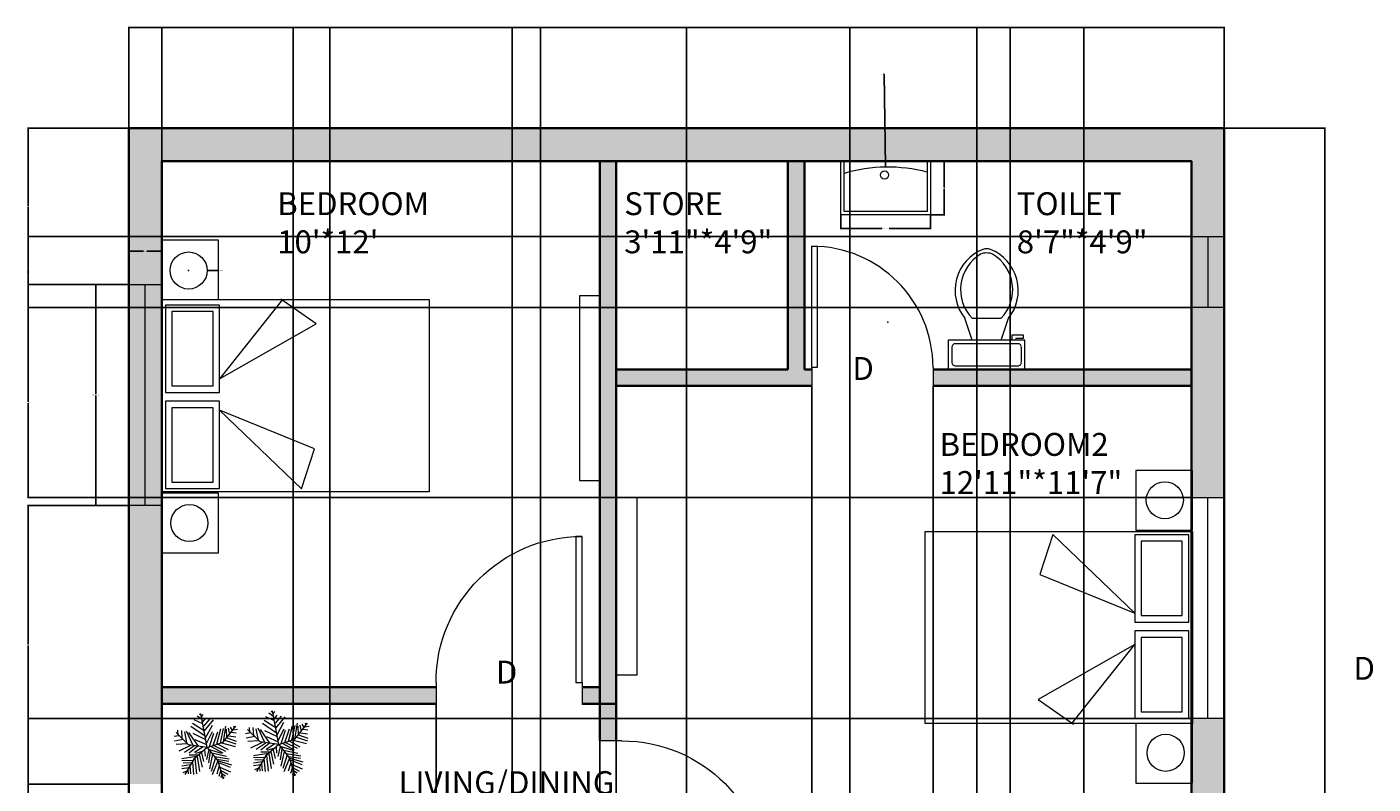
# Model space of a CAD drawing. Units: inches. Extents: x 1841 to 2210, y 2173 to 2736.
# Tile 4 of 4: x 1841 to 2210, y 2529 to 2736. Entities that reach past the tile are written whole.
import ezdxf

# ---------------------------------------------------------------- set-up
doc = ezdxf.new("R2010")
doc.units = ezdxf.units.IN
for name, color, linetype, lineweight in [('A-ANNO-DIMS', 2, 'Continuous', 18), ('A-AREA-IDEN', 10, 'Continuous', 18), ('A-FLOR-FIXT', 9, 'Continuous', 18), ('A-FURN', 8, 'Continuous', 18), ('A-WALL', 7, 'Continuous', 35), ('A-WALL-PATT', 252, 'Continuous', 13), ('BED', 120, 'Continuous', 18), ('DOOR', 50, 'Continuous', 18), ('TEXT', 10, 'Continuous', 18), ('TREE', 70, 'Continuous', 13), ('WIN', 193, 'Continuous', 18)]:
    doc.layers.add(name, color=color, linetype=linetype, lineweight=lineweight)
doc.styles.get("Standard").update_dxf_attribs({"font": 'arial.ttf'})
doc.dimstyles.get("Standard").update_dxf_attribs({"dimtxt": 0.18, "dimasz": 0.18, "dimexe": 0.18, "dimexo": 0.0625, "dimgap": 0.09, "dimtad": 0, "dimtih": 1, "dimtoh": 1, "dimdec": 4, "dimzin": 0, "dimdsep": 46, "dimtxsty": 'Standard', "dimcen": 0.09, "dimadec": 0, "dimazin": 0, "dimtfac": 1, "dimtdec": 4, "dimtofl": 0, "dimtmove": 0, "dimatfit": 3, "dimfxl": 1, "dimtolj": 1, "dimtzin": 0, "dimarcsym": 0})

# ---------------------------------------------------------------- blocks, each defined once
blk = doc.blocks.new('*U2')
for p, q in [((0, 0), (0, -6)), ((40, 0), (40, -6))]:
    blk.add_line(p, q)
blk.add_lwpolyline([(0, 0), (0, 40), (1.75, 40), (1.75, 0)], close=True)
blk.add_arc((0, 0), 40, 0, 90)
blk = doc.blocks.new('*U4')
for p, q in [((9.5, -6), (9.5, -2)), ((-10, -8.5), (-8, -8.5)), ((-10, -9.5), (-10, -8.5)), ((-7, -9.5), (-10, -9.5)), ((-8, -8.5), (-8, -8)), ((-7, -8), (-7, -9.5)), ((-4, -8), (-6, -14)), ((4, -8), (6, -14)), ((4, -14), (-4, -14))]:
    blk.add_line(p, q)
blk.add_lwpolyline([(10.5, -8), (10.5, 0), (-10.5, 0), (-10.5, -8)], close=True)
for points in [[(-9.5, -2), (-9.5, -6)], [(8.5, -1), (-8.5, -1)], [(-8.5, -7), (8.5, -7)]]:
    blk.add_lwpolyline(points)
for centre, radius, start, end in [((-8.62, -1.88), 0.884, 81.8699, 188.1301), ((8.62, -1.88), 0.884, 351.8699, 98.1301), ((-8.62, -6.12), 0.884, 171.8699, 278.1301), ((8.62, -6.12), 0.884, 261.8699, 8.1301), ((3.52, -21.58), 12.17, 141.4691, 247.9714), ((4.2, -21.82), 11.33, 136.3677, 238.9468), ((-3.52, -21.58), 12.17, 292.0284, 38.5307), ((-4.2, -21.82), 11.33, 301.053, 43.6321), ((0, -27.88), 4, 245.7318, 294.2682), ((0, -29), 4, 254.8605, 285.1395)]:
    blk.add_arc(centre, radius, start, end)
blk = doc.blocks.new('*U6')
for p, q in [((-7.288, 39.707), (-21.778, 46.673)), ((-8.737, 47.138), (-17.069, 52.711)), ((-10.186, 53.64), (-13.084, 55.962)), ((0, 0), (-10.5, 57)), ((-9.099, 51.782), (-6.563, 55.962)), ((-7.65, 43.423), (-2.578, 49.46)), ((-5.839, 35.992), (4.667, 48.067)), ((-5.114, 27.632), (10.463, 46.673)), ((-31.5, 4.5), (-52.5, 25.5)), ((-48.585, 21.131), (-49.309, 29.026)), ((-43.513, 28.561), (-42.427, 15.558)), ((-38.442, 26.239), (-34.819, 7.663)), ((-35.544, 28.097), (-24.314, 3.947)), ((-14.533, 2.09), (-30.834, 25.31)), ((-3.665, 19.273), (-27.574, 35.527)), ((-5.114, 28.097), (-24.676, 40.636)), ((-24.314, 23.917), (-2.941, 13.7)), ((-2.941, 16.486), (8.652, 37.85)), ((-1.129, 6.734), (9.014, 26.704)), ((3.942, 1.625), (11.187, 24.381)), ((10.101, 3.483), (17.708, 26.239)), ((16.259, 5.805), (23.142, 31.348)), ((22.055, 7.198), (27.489, 32.277)), ((27, 9), (48, 36)), ((27.127, 9.056), (31.112, 35.992)), ((31.836, 30.883), (32.561, 16.486)), ((35.096, 32.741), (37.27, 22.524)), ((38.719, 34.134), (41.979, 28.561)), ((40.53, 25.775), (48.862, 24.846)), ((43.791, 29.954), (51.036, 30.883)), ((44.153, 36.456), (45.239, 32.741)), ((-47.498, 19.737), (-55.83, 18.344)), ((-40.615, 13.7), (-55.105, 10.913)), ((-33.37, 6.269), (-52.207, 5.34)), ((-28.299, 3.483), (-47.86, -5.805)), ((-21.416, 3.018), (-38.079, -8.128)), ((0, 0), (-31.5, 4.5)), ((-15.982, 2.09), (-30.11, -9.521)), ((0, 0), (-22.5, -19.5)), ((-6.563, 1.161), (-21.416, -8.128)), ((-20.691, 13.7), (-1.129, 4.876)), ((0, 0), (27, 9)), ((0, 0), (18, -22.5)), ((6.478, 1.625), (26.04, -8.592)), ((11.187, 3.483), (30.749, -5.805)), ((18.07, 5.805), (35.096, -3.483)), ((24.229, 7.663), (46.688, 1.625)), ((29.662, 12.307), (48.137, 6.269)), ((33.285, 16.486), (48.862, 10.913)), ((36.183, 19.737), (48.137, 17.88)), ((-17.431, -15.094), (-42.789, -18.809)), ((-24.314, -21.596), (-42.427, -22.06)), ((-22.5, -19.5), (-37.5, -45)), ((-15.257, -12.772), (-30.11, -12.772)), ((-20.691, -18.345), (-17.793, -44.352)), ((-6.563, -5.805), (-19.967, -9.985)), ((-17.069, -15.094), (-12.721, -40.172)), ((-13.446, -11.378), (-8.737, -32.741)), ((-9.461, -8.592), (-6.201, -23.453)), ((-4.752, -3.483), (-3.665, -14.629)), ((2.493, -3.019), (-1.491, -20.202)), ((1.769, -2.555), (24.229, -9.521)), ((5.029, -6.27), (2.131, -25.775)), ((9.014, -11.378), (3.58, -35.992)), ((14.085, -16.951), (6.478, -40.172)), ((7.565, -9.056), (32.198, -14.629)), ((18.07, -22.524), (8.289, -45.745)), ((12.274, -15.094), (36.907, -18.809)), ((16.259, -19.738), (36.183, -22.989)), ((18, -22.5), (27, -52.5)), ((18.433, -22.524), (40.53, -29.026)), ((-28.299, -29.026), (-42.789, -31.348)), ((-30.834, -34.135), (-42.427, -35.528)), ((-34.457, -39.708), (-40.978, -42.494)), ((-26.849, -26.24), (-40.253, -25.775)), ((-32.646, -36.921), (-31.921, -44.352)), ((-29.023, -30.884), (-27.936, -43.887)), ((-25.038, -23.918), (-22.865, -45.281)), ((20.244, -30.419), (15.897, -44.816)), ((19.157, -25.311), (38.719, -33.206)), ((22.78, -37.85), (19.519, -48.532)), ((21.331, -32.741), (39.081, -40.636)), ((22.78, -38.314), (34.372, -44.816)), ((24.591, -43.423), (30.749, -47.603)), ((24.591, -45.745), (23.142, -50.854)), ((26.764, -49.925), (28.213, -50.854))]:
    blk.add_line(p, q)
blk = doc.blocks.new('BED-DOUBLE-WITH-NIGHTSTANDS')
for p, q in [((33.07, 69.27), (15.79, 47.62)), ((42.3, 62.7), (32.63, 69.37)), ((15.79, 47.62), (42.3, 62.7)), ((15.79, 39), (38.26, 17.46)), ((41.84, 28.47), (15.79, 39)), ((38.26, 17.46), (41.84, 28.47))]:
    blk.add_line(p, q)
for points in [[(0, 69.27), (15.55, 69.27), (15.55, 85.57), (0, 85.57)], [(0, 69.27), (73.23, 69.27), (73.23, 16.72), (0, 16.72)], [(1.03, 43.89), (15.79, 43.89), (15.79, 67.76), (1.03, 67.76)], [(2.79, 45.65), (14.04, 45.65), (14.04, 66), (2.79, 66)], [(1.03, 17.59), (15.79, 17.59), (15.79, 41.47), (1.03, 41.47)], [(2.79, 19.35), (14.04, 19.35), (14.04, 39.71), (2.79, 39.71)], [(0, 0), (15.55, 0), (15.55, 16.3), (0, 16.3)]]:
    blk.add_lwpolyline(points, close=True)
for centre in [(7.36, 77.24), (7.58, 8.12)]:
    blk.add_circle(centre, 5.08)
blk = doc.blocks.new('WIN-60IN-NOM')
blk.add_line((4.5, 0), (4.5, 60.52))
blk.add_lwpolyline([(0, 60.52), (9, 60.52), (9, 0), (0, 0)], close=True)
blk = doc.blocks.new('BASIN-WALL')
blk.add_lwpolyline([(24.58, 14.71), (24.58, 0), (0, 0), (0, 14.71)])
blk.add_lwpolyline([(0.91, 14.71), (23.68, 14.71), (23.68, 0.91), (0.91, 0.91)], close=True)
blk.add_circle((11.97, 10.91), 1.13)
blk.add_arc((12.85, -29.32), 42.4, 75.2054, 106.3847)
blk = doc.blocks.new('*D12')
at = {"layer": 'A-ANNO-DIMS', "color": 0, "lineweight": -2, "transparency": 16777216}
for p, q in [((1868.99, 2665.67), (1859.79, 2665.67)), ((1859.97, 2665.49), (1859.97, 2635.59)), ((1859.97, 2605.33), (1859.97, 2635.23)), ((1868.99, 2605.15), (1859.79, 2605.15))]:
    blk.add_line(p, q, dxfattribs=at)
at = {"layer": 'A-ANNO-DIMS', "color": 0, "transparency": 16777216}
for points in [[(1859.94, 2665.49), (1860, 2665.49), (1859.97, 2665.67)], [(1859.94, 2605.33), (1860, 2605.33), (1859.97, 2605.15)]]:
    blk.add_solid(points, dxfattribs=at)
at = {"layer": 'Defpoints', "color": 0, "transparency": 16777216}
for p in [(1859.97, 2665.67), (1869.05, 2665.67), (1869.05, 2605.15)]:
    blk.add_point(p, dxfattribs=at)
at = {"layer": 'A-ANNO-DIMS', "color": 0, "transparency": 16777216, "insert": (1859.97, 2635.41), "char_height": 0.18, "attachment_point": 5}
blk.add_mtext('\\A1;WINDOW 61 TYP.', dxfattribs=at)
blk = doc.blocks.new('*D13')
at = {"layer": 'A-ANNO-DIMS', "color": 0, "lineweight": -2, "transparency": 16777216}
for p, q in [((1869.05, 2665.73), (1869.05, 2674.93)), ((1869.23, 2674.75), (1873.09, 2674.75)), ((1877.87, 2674.75), (1874.01, 2674.75)), ((1878.05, 2665.73), (1878.05, 2674.93))]:
    blk.add_line(p, q, dxfattribs=at)
at = {"layer": 'A-ANNO-DIMS', "color": 0, "transparency": 16777216}
for points in [[(1869.23, 2674.78), (1869.23, 2674.72), (1869.05, 2674.75)], [(1877.87, 2674.78), (1877.87, 2674.72), (1878.05, 2674.75)]]:
    blk.add_solid(points, dxfattribs=at)
at = {"layer": 'Defpoints', "color": 0, "transparency": 16777216}
for p in [(1878.05, 2674.75), (1869.05, 2665.67), (1878.05, 2665.67)]:
    blk.add_point(p, dxfattribs=at)
at = {"layer": 'A-ANNO-DIMS', "color": 0, "transparency": 16777216, "insert": (1873.55, 2674.75), "char_height": 0.18, "attachment_point": 5}
blk.add_mtext('\\A1;9 TYP.', dxfattribs=at)
blk = doc.blocks.new('*D20')
at = {"layer": 'A-ANNO-DIMS', "color": 0, "lineweight": -2, "transparency": 16777216}
for p, q in [((2064.03, 2684.63), (2064.03, 2680.83)), ((2088.61, 2684.63), (2088.61, 2680.83)), ((2064.21, 2681.01), (2075.39, 2681.01)), ((2088.43, 2681.01), (2077.26, 2681.01))]:
    blk.add_line(p, q, dxfattribs=at)
at = {"layer": 'A-ANNO-DIMS', "color": 0, "transparency": 16777216}
for points in [[(2064.21, 2681.04), (2064.21, 2680.98), (2064.03, 2681.01)], [(2088.43, 2681.04), (2088.43, 2680.98), (2088.61, 2681.01)]]:
    blk.add_solid(points, dxfattribs=at)
at = {"layer": 'Defpoints', "color": 0, "transparency": 16777216}
for p in [(2064.03, 2684.69), (2088.61, 2684.69), (2088.61, 2681.01)]:
    blk.add_point(p, dxfattribs=at)
at = {"layer": 'A-ANNO-DIMS', "color": 0, "transparency": 16777216, "insert": (2076.32, 2681.01), "char_height": 0.18, "attachment_point": 5}
blk.add_mtext('\\A1;BASIN 25 TYP.', dxfattribs=at)
blk = doc.blocks.new('*D21')
at = {"layer": 'A-ANNO-DIMS', "color": 0, "lineweight": -2, "transparency": 16777216}
for p, q in [((2088.68, 2699.41), (2092.48, 2699.41)), ((2092.3, 2699.23), (2092.3, 2692.23)), ((2092.3, 2684.87), (2092.3, 2691.87)), ((2088.68, 2684.69), (2092.48, 2684.69))]:
    blk.add_line(p, q, dxfattribs=at)
at = {"layer": 'A-ANNO-DIMS', "color": 0, "transparency": 16777216}
for points in [[(2092.27, 2699.23), (2092.33, 2699.23), (2092.3, 2699.41)], [(2092.27, 2684.87), (2092.33, 2684.87), (2092.3, 2684.69)]]:
    blk.add_solid(points, dxfattribs=at)
at = {"layer": 'Defpoints', "color": 0, "transparency": 16777216}
for p in [(2088.61, 2699.41), (2092.3, 2699.41), (2088.61, 2684.69)]:
    blk.add_point(p, dxfattribs=at)
at = {"layer": 'A-ANNO-DIMS', "color": 0, "transparency": 16777216, "insert": (2092.3, 2692.05), "char_height": 0.18, "attachment_point": 5}
blk.add_mtext('\\A1;15 TYP.', dxfattribs=at)
blk = doc.blocks.new('*D22')
at = {"layer": 'A-ANNO-DIMS', "color": 0, "lineweight": -2, "transparency": 16777216}
for p, q in [((1869.05, 2708.47), (1869.05, 2736.14)), ((1869.23, 2735.96), (2018.76, 2735.96)), ((2168.87, 2735.96), (2019.34, 2735.96)), ((2169.05, 2708.47), (2169.05, 2736.14))]:
    blk.add_line(p, q, dxfattribs=at)
at = {"layer": 'A-ANNO-DIMS', "color": 0, "transparency": 16777216}
for points in [[(1869.23, 2735.99), (1869.23, 2735.93), (1869.05, 2735.96)], [(2168.87, 2735.99), (2168.87, 2735.93), (2169.05, 2735.96)]]:
    blk.add_solid(points, dxfattribs=at)
at = {"layer": 'Defpoints', "color": 0, "transparency": 16777216}
for p in [(2169.05, 2735.96), (1869.05, 2708.41), (2169.05, 2708.41)]:
    blk.add_point(p, dxfattribs=at)
at = {"layer": 'A-ANNO-DIMS', "color": 0, "transparency": 16777216, "insert": (2019.05, 2735.96), "char_height": 0.18, "attachment_point": 5}
blk.add_mtext('\\A1;300', dxfattribs=at)
blk = doc.blocks.new('*D23')
at = {"layer": 'A-ANNO-DIMS', "color": 0, "lineweight": -2, "transparency": 16777216}
for p, q in [((2169.11, 2708.41), (2196.78, 2708.41)), ((2196.6, 2708.23), (2196.6, 2458.59)), ((2196.6, 2208.59), (2196.6, 2458.22)), ((2028.61, 2208.41), (2196.78, 2208.41))]:
    blk.add_line(p, q, dxfattribs=at)
at = {"layer": 'A-ANNO-DIMS', "color": 0, "transparency": 16777216}
for points in [[(2196.57, 2708.23), (2196.63, 2708.23), (2196.6, 2708.41)], [(2196.57, 2208.59), (2196.63, 2208.59), (2196.6, 2208.41)]]:
    blk.add_solid(points, dxfattribs=at)
at = {"layer": 'Defpoints', "color": 0, "transparency": 16777216}
for p in [(2169.05, 2708.41), (2196.6, 2708.41), (2028.55, 2208.41)]:
    blk.add_point(p, dxfattribs=at)
at = {"layer": 'A-ANNO-DIMS', "color": 0, "transparency": 16777216, "insert": (2196.6, 2458.41), "char_height": 0.18, "attachment_point": 5}
blk.add_mtext('\\A1;500', dxfattribs=at)
blk = doc.blocks.new('*D31')
at = {"layer": 'A-ANNO-DIMS', "color": 0, "lineweight": -2, "transparency": 16777216}
for p, q in [((1868.99, 2605.15), (1841.32, 2605.15)), ((1841.5, 2604.97), (1841.5, 2567.22)), ((1841.5, 2529.1), (1841.5, 2566.86)), ((1868.99, 2528.92), (1841.32, 2528.92))]:
    blk.add_line(p, q, dxfattribs=at)
at = {"layer": 'A-ANNO-DIMS', "color": 0, "transparency": 16777216}
for points in [[(1841.47, 2604.97), (1841.53, 2604.97), (1841.5, 2605.15)], [(1841.47, 2529.1), (1841.53, 2529.1), (1841.5, 2528.92)]]:
    blk.add_solid(points, dxfattribs=at)
at = {"layer": 'Defpoints', "color": 0, "transparency": 16777216}
for p in [(1841.5, 2605.15), (1869.05, 2605.15), (1869.05, 2528.92)]:
    blk.add_point(p, dxfattribs=at)
at = {"layer": 'A-ANNO-DIMS', "color": 0, "transparency": 16777216, "insert": (1841.5, 2567.04), "char_height": 0.18, "attachment_point": 5}
blk.add_mtext('\\A1;76.23', dxfattribs=at)
blk = doc.blocks.new('*D32')
at = {"layer": 'A-ANNO-DIMS', "color": 0, "lineweight": -2, "transparency": 16777216}
for p, q in [((1868.99, 2708.41), (1841.32, 2708.41)), ((1841.5, 2708.23), (1841.5, 2687.22)), ((1841.5, 2665.85), (1841.5, 2686.86)), ((1868.99, 2665.67), (1841.32, 2665.67))]:
    blk.add_line(p, q, dxfattribs=at)
at = {"layer": 'A-ANNO-DIMS', "color": 0, "transparency": 16777216}
for points in [[(1841.47, 2708.23), (1841.53, 2708.23), (1841.5, 2708.41)], [(1841.47, 2665.85), (1841.53, 2665.85), (1841.5, 2665.67)]]:
    blk.add_solid(points, dxfattribs=at)
at = {"layer": 'Defpoints', "color": 0, "transparency": 16777216}
for p in [(1841.5, 2708.41), (1869.05, 2708.41), (1869.05, 2665.67)]:
    blk.add_point(p, dxfattribs=at)
at = {"layer": 'A-ANNO-DIMS', "color": 0, "transparency": 16777216, "insert": (1841.5, 2687.04), "char_height": 0.18, "attachment_point": 5}
blk.add_mtext('\\A1;42.736', dxfattribs=at)
blk = doc.blocks.new('*D33')
at = {"layer": 'A-ANNO-DIMS', "color": 0, "lineweight": -2, "transparency": 16777216}
for p, q in [((2159.99, 2678.81), (1841.32, 2678.81)), ((1841.5, 2678.63), (1841.5, 2669.27)), ((1841.5, 2659.54), (1841.5, 2668.91)), ((2159.99, 2659.36), (1841.32, 2659.36))]:
    blk.add_line(p, q, dxfattribs=at)
at = {"layer": 'A-ANNO-DIMS', "color": 0, "transparency": 16777216}
for points in [[(1841.47, 2678.63), (1841.53, 2678.63), (1841.5, 2678.81)], [(1841.47, 2659.54), (1841.53, 2659.54), (1841.5, 2659.36)]]:
    blk.add_solid(points, dxfattribs=at)
at = {"layer": 'Defpoints', "color": 0, "transparency": 16777216}
for p in [(2160.05, 2678.81), (1841.5, 2659.36), (2160.05, 2659.36)]:
    blk.add_point(p, dxfattribs=at)
at = {"layer": 'A-ANNO-DIMS', "color": 0, "transparency": 16777216, "insert": (1841.5, 2669.09), "char_height": 0.18, "attachment_point": 5}
blk.add_mtext('\\A1;19.448', dxfattribs=at)
blk = doc.blocks.new('*D34')
at = {"layer": 'A-ANNO-DIMS', "color": 0, "lineweight": -2, "transparency": 16777216}
for p, q in [((2159.99, 2659.36), (1841.32, 2659.36)), ((1841.5, 2659.18), (1841.5, 2633.53)), ((1841.5, 2607.52), (1841.5, 2633.17)), ((2159.99, 2607.34), (1841.32, 2607.34))]:
    blk.add_line(p, q, dxfattribs=at)
at = {"layer": 'A-ANNO-DIMS', "color": 0, "transparency": 16777216}
for points in [[(1841.47, 2659.18), (1841.53, 2659.18), (1841.5, 2659.36)], [(1841.47, 2607.52), (1841.53, 2607.52), (1841.5, 2607.34)]]:
    blk.add_solid(points, dxfattribs=at)
at = {"layer": 'Defpoints', "color": 0, "transparency": 16777216}
for p in [(1841.5, 2659.36), (2160.05, 2659.36), (2160.05, 2607.34)]:
    blk.add_point(p, dxfattribs=at)
at = {"layer": 'A-ANNO-DIMS', "color": 0, "transparency": 16777216, "insert": (1841.5, 2633.35), "char_height": 0.18, "attachment_point": 5}
blk.add_mtext('\\A1;52.03', dxfattribs=at)
blk = doc.blocks.new('*D35')
at = {"layer": 'A-ANNO-DIMS', "color": 0, "lineweight": -2, "transparency": 16777216}
for p, q in [((2159.99, 2546.82), (1841.32, 2546.82)), ((1841.5, 2546.64), (1841.5, 2523.04)), ((1841.5, 2499.09), (1841.5, 2522.68)), ((2159.99, 2498.91), (1841.32, 2498.91))]:
    blk.add_line(p, q, dxfattribs=at)
at = {"layer": 'A-ANNO-DIMS', "color": 0, "transparency": 16777216}
for points in [[(1841.47, 2546.64), (1841.53, 2546.64), (1841.5, 2546.82)], [(1841.47, 2499.09), (1841.53, 2499.09), (1841.5, 2498.91)]]:
    blk.add_solid(points, dxfattribs=at)
at = {"layer": 'Defpoints', "color": 0, "transparency": 16777216}
for p in [(1841.5, 2546.82), (2160.05, 2546.82), (2160.05, 2498.91)]:
    blk.add_point(p, dxfattribs=at)
at = {"layer": 'A-ANNO-DIMS', "color": 0, "transparency": 16777216, "insert": (1841.5, 2522.86), "char_height": 0.18, "attachment_point": 5}
blk.add_mtext('\\A1;47.91', dxfattribs=at)
blk = doc.blocks.new('*D36')
at = {"layer": 'A-ANNO-DIMS', "color": 0, "lineweight": -2, "transparency": 16777216}
for p, q in [((1981.8, 2316.47), (1981.8, 2736.14)), ((1981.98, 2735.96), (2001.58, 2735.96)), ((2021.62, 2735.96), (2002.02, 2735.96)), ((2021.8, 2316.47), (2021.8, 2736.14))]:
    blk.add_line(p, q, dxfattribs=at)
at = {"layer": 'A-ANNO-DIMS', "color": 0, "transparency": 16777216}
for points in [[(1981.98, 2735.99), (1981.98, 2735.93), (1981.8, 2735.96)], [(2021.62, 2735.99), (2021.62, 2735.93), (2021.8, 2735.96)]]:
    blk.add_solid(points, dxfattribs=at)
at = {"layer": 'Defpoints', "color": 0, "transparency": 16777216}
for p in [(2021.8, 2735.96), (1981.8, 2316.41), (2021.8, 2316.41)]:
    blk.add_point(p, dxfattribs=at)
at = {"layer": 'A-ANNO-DIMS', "color": 0, "transparency": 16777216, "insert": (2001.8, 2735.96), "char_height": 0.18, "attachment_point": 5}
blk.add_mtext('\\A1;40', dxfattribs=at)
blk = doc.blocks.new('*D37')
at = {"layer": 'A-ANNO-DIMS', "color": 0, "lineweight": -2, "transparency": 16777216}
for p, q in [((1878.05, 2402.47), (1878.05, 2736.14)), ((1878.23, 2735.96), (1895.83, 2735.96)), ((1913.87, 2735.96), (1896.27, 2735.96)), ((1914.05, 2402.47), (1914.05, 2736.14))]:
    blk.add_line(p, q, dxfattribs=at)
at = {"layer": 'A-ANNO-DIMS', "color": 0, "transparency": 16777216}
for points in [[(1878.23, 2735.99), (1878.23, 2735.93), (1878.05, 2735.96)], [(1913.87, 2735.99), (1913.87, 2735.93), (1914.05, 2735.96)]]:
    blk.add_solid(points, dxfattribs=at)
at = {"layer": 'Defpoints', "color": 0, "transparency": 16777216}
for p in [(1914.05, 2735.96), (1878.05, 2402.41), (1914.05, 2402.41)]:
    blk.add_point(p, dxfattribs=at)
at = {"layer": 'A-ANNO-DIMS', "color": 0, "transparency": 16777216, "insert": (1896.05, 2735.96), "char_height": 0.18, "attachment_point": 5}
blk.add_mtext('\\A1;36', dxfattribs=at)
blk = doc.blocks.new('*D38')
at = {"layer": 'A-ANNO-DIMS', "color": 0, "lineweight": -2, "transparency": 16777216}
for p, q in [((1914.05, 2352.47), (1914.05, 2736.14)), ((1914.23, 2735.96), (1943.83, 2735.96)), ((1973.87, 2735.96), (1944.27, 2735.96)), ((1974.05, 2352.47), (1974.05, 2736.14))]:
    blk.add_line(p, q, dxfattribs=at)
at = {"layer": 'A-ANNO-DIMS', "color": 0, "transparency": 16777216}
for points in [[(1914.23, 2735.99), (1914.23, 2735.93), (1914.05, 2735.96)], [(1973.87, 2735.99), (1973.87, 2735.93), (1974.05, 2735.96)]]:
    blk.add_solid(points, dxfattribs=at)
at = {"layer": 'Defpoints', "color": 0, "transparency": 16777216}
for p in [(1974.05, 2735.96), (1914.05, 2352.41), (1974.05, 2352.41)]:
    blk.add_point(p, dxfattribs=at)
at = {"layer": 'A-ANNO-DIMS', "color": 0, "transparency": 16777216, "insert": (1944.05, 2735.96), "char_height": 0.18, "attachment_point": 5}
blk.add_mtext('\\A1;60', dxfattribs=at)
blk = doc.blocks.new('*D42')
at = {"layer": 'A-ANNO-DIMS', "color": 0, "lineweight": -2, "transparency": 16777216}
for p, q in [((1878.05, 2550.84), (1878.05, 2180.68)), ((1953.17, 2550.84), (1953.17, 2180.68)), ((1878.23, 2180.86), (1915.22, 2180.86)), ((1952.99, 2180.86), (1916, 2180.86))]:
    blk.add_line(p, q, dxfattribs=at)
at = {"layer": 'A-ANNO-DIMS', "color": 0, "transparency": 16777216}
for points in [[(1878.23, 2180.89), (1878.23, 2180.83), (1878.05, 2180.86)], [(1952.99, 2180.89), (1952.99, 2180.83), (1953.17, 2180.86)]]:
    blk.add_solid(points, dxfattribs=at)
at = {"layer": 'Defpoints', "color": 0, "transparency": 16777216}
for p in [(1878.05, 2550.91), (1953.17, 2550.91), (1953.17, 2180.86)]:
    blk.add_point(p, dxfattribs=at)
at = {"layer": 'A-ANNO-DIMS', "color": 0, "transparency": 16777216, "insert": (1915.61, 2180.86), "char_height": 0.18, "attachment_point": 5}
blk.add_mtext('\\A1;75.12', dxfattribs=at)
blk = doc.blocks.new('*D43')
at = {"layer": 'A-ANNO-DIMS', "color": 0, "lineweight": -2, "transparency": 16777216}
for p, q in [((2056.06, 2637.84), (2056.06, 2180.68)), ((2089.3, 2637.84), (2089.3, 2180.68)), ((2056.24, 2180.86), (2072.22, 2180.86)), ((2089.12, 2180.86), (2073.14, 2180.86))]:
    blk.add_line(p, q, dxfattribs=at)
at = {"layer": 'A-ANNO-DIMS', "color": 0, "transparency": 16777216}
for points in [[(2056.24, 2180.89), (2056.24, 2180.83), (2056.06, 2180.86)], [(2089.12, 2180.89), (2089.12, 2180.83), (2089.3, 2180.86)]]:
    blk.add_solid(points, dxfattribs=at)
at = {"layer": 'Defpoints', "color": 0, "transparency": 16777216}
for p in [(2056.06, 2637.91), (2089.3, 2637.91), (2089.3, 2180.86)]:
    blk.add_point(p, dxfattribs=at)
at = {"layer": 'A-ANNO-DIMS', "color": 0, "transparency": 16777216, "insert": (2072.68, 2180.86), "char_height": 0.18, "attachment_point": 5}
blk.add_mtext('\\A1;33.234', dxfattribs=at)
blk = doc.blocks.new('*D45')
at = {"layer": 'A-ANNO-DIMS', "color": 0, "lineweight": -2, "transparency": 16777216}
for p, q in [((1998.05, 2540.69), (1998.05, 2180.68)), ((2002.55, 2540.69), (2002.55, 2180.68)), ((1998.23, 2180.86), (2000.04, 2180.86)), ((2002.37, 2180.86), (2000.56, 2180.86))]:
    blk.add_line(p, q, dxfattribs=at)
at = {"layer": 'A-ANNO-DIMS', "color": 0, "transparency": 16777216}
for points in [[(1998.23, 2180.89), (1998.23, 2180.83), (1998.05, 2180.86)], [(2002.37, 2180.89), (2002.37, 2180.83), (2002.55, 2180.86)]]:
    blk.add_solid(points, dxfattribs=at)
at = {"layer": 'Defpoints', "color": 0, "transparency": 16777216}
for p in [(1998.05, 2540.75), (2002.55, 2540.75), (2002.55, 2180.86)]:
    blk.add_point(p, dxfattribs=at)
at = {"layer": 'A-ANNO-DIMS', "color": 0, "transparency": 16777216, "insert": (2000.3, 2180.86), "char_height": 0.18, "attachment_point": 5}
blk.add_mtext('\\A1;4.5', dxfattribs=at)
blk = doc.blocks.new('*D46')
at = {"layer": 'A-ANNO-DIMS', "color": 0, "lineweight": -2, "transparency": 16777216}
for p, q in [((1914.05, 2316.47), (1914.05, 2736.14)), ((1914.23, 2735.96), (1918.84, 2735.96)), ((1923.87, 2735.96), (1919.26, 2735.96)), ((1924.05, 2316.47), (1924.05, 2736.14))]:
    blk.add_line(p, q, dxfattribs=at)
at = {"layer": 'A-ANNO-DIMS', "color": 0, "transparency": 16777216}
for points in [[(1914.23, 2735.99), (1914.23, 2735.93), (1914.05, 2735.96)], [(1923.87, 2735.99), (1923.87, 2735.93), (1924.05, 2735.96)]]:
    blk.add_solid(points, dxfattribs=at)
at = {"layer": 'Defpoints', "color": 0, "transparency": 16777216}
for p in [(1924.05, 2735.96), (1914.05, 2316.41), (1924.05, 2316.41)]:
    blk.add_point(p, dxfattribs=at)
at = {"layer": 'A-ANNO-DIMS', "color": 0, "transparency": 16777216, "insert": (1919.05, 2735.96), "char_height": 0.18, "attachment_point": 5}
blk.add_mtext('\\A1;10', dxfattribs=at)
blk = doc.blocks.new('*D47')
at = {"layer": 'A-ANNO-DIMS', "color": 0, "lineweight": -2, "transparency": 16777216}
for p, q in [((2066.54, 2442.55), (2066.54, 2736.14)), ((2066.72, 2735.96), (2083.52, 2735.96)), ((2101.11, 2735.96), (2084.31, 2735.96)), ((2101.29, 2442.55), (2101.29, 2736.14))]:
    blk.add_line(p, q, dxfattribs=at)
at = {"layer": 'A-ANNO-DIMS', "color": 0, "transparency": 16777216}
for points in [[(2066.72, 2735.99), (2066.72, 2735.93), (2066.54, 2735.96)], [(2101.11, 2735.99), (2101.11, 2735.93), (2101.29, 2735.96)]]:
    blk.add_solid(points, dxfattribs=at)
at = {"layer": 'Defpoints', "color": 0, "transparency": 16777216}
for p in [(2101.29, 2735.96), (2066.54, 2442.49), (2101.29, 2442.49)]:
    blk.add_point(p, dxfattribs=at)
at = {"layer": 'A-ANNO-DIMS', "color": 0, "transparency": 16777216, "insert": (2083.91, 2735.96), "char_height": 0.18, "attachment_point": 5}
blk.add_mtext('\\A1;34.75', dxfattribs=at)
blk = doc.blocks.new('*D49')
at = {"layer": 'A-ANNO-DIMS', "color": 0, "lineweight": -2, "transparency": 16777216}
for p, q in [((2110.38, 2487.94), (2110.38, 2736.14)), ((2110.56, 2735.96), (2120.1, 2735.96)), ((2130.41, 2735.96), (2120.86, 2735.96)), ((2130.59, 2487.94), (2130.59, 2736.14))]:
    blk.add_line(p, q, dxfattribs=at)
at = {"layer": 'A-ANNO-DIMS', "color": 0, "transparency": 16777216}
for points in [[(2110.56, 2735.99), (2110.56, 2735.93), (2110.38, 2735.96)], [(2130.41, 2735.99), (2130.41, 2735.93), (2130.59, 2735.96)]]:
    blk.add_solid(points, dxfattribs=at)
at = {"layer": 'Defpoints', "color": 0, "transparency": 16777216}
for p in [(2130.59, 2735.96), (2110.38, 2487.88), (2130.59, 2487.88)]:
    blk.add_point(p, dxfattribs=at)
at = {"layer": 'A-ANNO-DIMS', "color": 0, "transparency": 16777216, "insert": (2120.48, 2735.96), "char_height": 0.18, "attachment_point": 5}
blk.add_mtext('\\A1;20.21', dxfattribs=at)
blk = doc.blocks.new('*D52')
at = {"layer": 'A-ANNO-DIMS', "color": 0, "lineweight": -2, "transparency": 16777216}
for p, q in [((1885.32, 2669.46), (1885.5, 2669.46)), ((1885.41, 2669.37), (1885.41, 2669.55)), ((1893.53, 2669.46), (1890.67, 2669.46))]:
    blk.add_line(p, q, dxfattribs=at)
at = {"layer": 'A-ANNO-DIMS', "color": 0, "transparency": 16777216}
blk.add_solid([(1890.67, 2669.49), (1890.67, 2669.43), (1890.49, 2669.46)], dxfattribs=at)
at = {"layer": 'Defpoints', "color": 0, "transparency": 16777216}
for p in [(1880.34, 2669.46), (1890.49, 2669.46)]:
    blk.add_point(p, dxfattribs=at)
at = {"layer": 'A-ANNO-DIMS', "color": 0, "transparency": 16777216, "insert": (1894.21, 2669.46), "char_height": 0.18, "attachment_point": 5}
blk.add_mtext('\\A1;6X ∅10.15', dxfattribs=at)
blk = doc.blocks.new('*D53')
at = {"layer": 'A-ANNO-DIMS', "color": 0, "lineweight": -2, "transparency": 16777216}
for p, q in [((2075.76, 2723.21), (2075.94, 2723.21)), ((2075.94, 2723.21), (2076.29, 2697.95)), ((2076.79, 2655.37), (2076.97, 2655.37)), ((2076.88, 2655.28), (2076.88, 2655.46))]:
    blk.add_line(p, q, dxfattribs=at)
at = {"layer": 'A-ANNO-DIMS', "color": 0, "transparency": 16777216}
blk.add_solid([(2076.32, 2697.95), (2076.26, 2697.95), (2076.29, 2697.77)], dxfattribs=at)
at = {"layer": 'Defpoints', "color": 0, "transparency": 16777216}
for p in [(2076.29, 2697.77), (2076.88, 2655.37)]:
    blk.add_point(p, dxfattribs=at)
at = {"layer": 'A-ANNO-DIMS', "color": 0, "transparency": 16777216, "insert": (2075.15, 2723.21), "char_height": 0.18, "attachment_point": 5}
blk.add_mtext('\\A1;2X R42.4', dxfattribs=at)

msp = doc.modelspace()

# ---------------------------------------------------------------- hatches: boundary and pattern name
at = {"layer": 'A-WALL-PATT'}
h = msp.add_hatch(color=256, dxfattribs=at)
h.dxf.hatch_style = 1
h.paths.add_polyline_path([(2169.0509, 2546.8192), (2160.3559, 2546.8192), (2160.3559, 2545.451), (2160.3559, 2529.1476), (2160.0509, 2237.4052), (2128.1686, 2237.4052), (2128.1686, 2228.4052), (2169.0509, 2228.4052)])
h.paths.add_polyline_path([(2067.6527, 2237.4052), (2028.5509, 2237.4052), (2028.5509, 2228.4052), (2067.6527, 2228.4052)])
h.paths.add_polyline_path([(2033.0509, 2321.9228), (2028.5509, 2321.9228), (2028.5509, 2237.4052), (2033.0509, 2237.4052)])
h.paths.add_polyline_path([(2160.0509, 2369.9052), (2052.0509, 2369.9052), (2052.0509, 2380.7227), (2047.5509, 2380.7227), (2047.5509, 2369.9052), (2028.5509, 2369.9052), (2028.5509, 2364.1588), (2028.5509, 2361.9228), (2033.0509, 2361.9228), (2033.0509, 2365.4052), (2050.3181, 2365.4052), (2160.0509, 2365.4052)])
h.paths.add_polyline_path([(1878.0509, 2346.5722), (1869.0509, 2346.5722), (1869.0509, 2228.4052), (1878.0509, 2228.4052), (1878.0509, 2237.4052)])
h.paths.add_polyline_path([(1981.8009, 2316.4052), (1878.0509, 2316.4052), (1878.0509, 2311.9052), (1981.8009, 2311.9052)])
h.paths.add_polyline_path([(1978.2584, 2442.9052), (1878.0509, 2442.9052), (1878.0509, 2438.4052), (1914.0509, 2438.4052), (1978.2584, 2438.4052)])
h.paths.add_polyline_path([(1878.0509, 2468.4052), (1869.0509, 2468.4052), (1869.0509, 2407.0881), (1878.0509, 2407.0881), (1878.0509, 2438.4052)])
h.paths.add_polyline_path([(2028.5509, 2442.9052), (2018.2584, 2442.9052), (2018.2584, 2438.4052), (2028.5509, 2438.4052)])
h.paths.add_polyline_path([(2131.5968, 2498.9052), (2002.5509, 2498.9052), (2002.5509, 2500.7487), (1998.0509, 2500.7487), (1998.0509, 2494.4052), (2131.5968, 2494.4052)])
h.paths.add_polyline_path([(2033.0509, 2489.9052), (2033.0509, 2494.4052), (2028.5509, 2494.4052), (2028.5509, 2489.9052), (2028.5509, 2417.9052), (2131.5509, 2417.9052), (2131.5509, 2422.4052), (2033.0509, 2422.4052), (2033.0294, 2446.4052)])
h.paths.add_polyline_path([(1953.1667, 2555.4052), (1878.0509, 2555.4052), (1878.0509, 2550.9052), (1953.1667, 2550.9052)], flags=17)
h.paths.add_polyline_path([(1878.0509, 2699.4052), (2160.0509, 2699.4052), (2160.0509, 2607.3351), (2169.0509, 2607.3351), (2169.0509, 2708.4052), (1869.0509, 2708.4052), (1869.0509, 2528.9211), (1878.0509, 2528.9211), (1878.0509, 2550.9052), (1878.0509, 2555.4052)])
h.paths.add_polyline_path([(1998.0509, 2555.4052), (1993.1667, 2555.4052), (1993.1667, 2550.9052), (1998.0509, 2550.9052)], flags=17)
h.paths.add_polyline_path([(2002.5509, 2550.9052), (1998.0509, 2550.9052), (1998.0509, 2540.7487), (2002.5509, 2540.7487)], flags=17)
h.paths.add_polyline_path([(2002.5509, 2576.8157), (2002.5509, 2607.2805), (2002.5509, 2699.4052), (1998.0509, 2699.4052), (1998.0509, 2555.4052), (1998.0509, 2550.9052), (2002.5509, 2550.9052)], flags=17)
h.paths.add_polyline_path([(2160.0509, 2642.4052), (2089.2965, 2642.4052), (2089.2965, 2637.9052), (2160.0509, 2637.9052)], flags=17)
h.paths.add_polyline_path([(2056.0629, 2642.4052), (2054.0509, 2642.4052), (2054.0509, 2699.4052), (2049.5509, 2699.4052), (2049.5509, 2642.4052), (2002.5509, 2642.4052), (2002.5509, 2637.9052), (2054.0509, 2637.9052), (2056.0629, 2637.9052)], flags=17)
h.paths.add_polyline_path([(1924.594, 2243.1802), (1965.0263, 2243.1802), (1965.0263, 2266.5581), (1924.594, 2266.5581)], flags=9)
h.paths.add_polyline_path([(2082.2056, 2327.2752), (2130.8731, 2327.2752), (2130.8731, 2350.6531), (2082.2056, 2350.6531)], flags=9)
h.paths.add_polyline_path([(2000.1077, 2344.9343), (2000.1077, 2400.666), (1976.7298, 2400.666), (1976.7298, 2344.9343)], flags=9)
h.paths.add_polyline_path([(2161.6353, 2440.9897), (2161.6353, 2476.9732), (2138.2574, 2476.9732), (2138.2574, 2440.9897)], flags=24)
h.paths.add_polyline_path([(2044.2273, 2462.409), (2085.775, 2462.409), (2085.775, 2485.7869), (2044.2273, 2485.7869)], flags=25)
h.paths.add_polyline_path([(1940.3738, 2512.1813), (2005.58, 2512.1813), (2005.58, 2535.5592), (1940.3738, 2535.5592)], flags=9)
h.paths.add_polyline_path([(2088.5551, 2604.7497), (2142.0901, 2604.7497), (2142.0901, 2628.1276), (2088.5551, 2628.1276)], flags=25)
h.paths.add_polyline_path([(2110.3045, 2670.6273), (2145.8692, 2670.6273), (2145.8692, 2694.0052), (2110.3045, 2694.0052)], flags=25)
h.paths.add_polyline_path([(2002.7596, 2670.6273), (2043.2176, 2670.6273), (2043.2176, 2694.0052), (2002.7596, 2694.0052)], flags=24)
h.paths.add_polyline_path([(1907.1501, 2670.6273), (1955.8175, 2670.6273), (1955.8175, 2694.0052), (1907.1501, 2694.0052)], flags=25)

# ---------------------------------------------------------------- linework, layer by layer
at = {"layer": 'A-FURN'}
for points in [[(1998.0509, 2662.5455), (1992.4589, 2662.5455), (1992.4589, 2612.0032), (1998.0509, 2612.0032)], [(2002.5509, 2558.7822), (2008.279, 2558.7822), (2008.279, 2607.2805), (2002.5509, 2607.2805)]]:
    msp.add_lwpolyline(points, close=True, dxfattribs=at)
at = {"layer": 'A-WALL'}
for p, q in [((1878.0509, 2699.4052), (1998.0509, 2699.4052)), ((1998.0509, 2699.4052), (1998.0509, 2555.4052)), ((2002.5509, 2699.4052), (2002.5509, 2550.9052)), ((2002.5509, 2699.4052), (2049.5509, 2699.4052)), ((2049.5509, 2699.4052), (2049.5509, 2642.4052)), ((2054.0509, 2699.4052), (2054.0509, 2642.4052)), ((2054.0509, 2699.4052), (2157.0509, 2699.4052)), ((2049.5509, 2642.4052), (2002.5509, 2642.4052)), ((2054.0509, 2642.4052), (2056.0629, 2642.4052)), ((2089.2965, 2642.4052), (2160.0509, 2642.4052)), ((2054.0509, 2637.9052), (2002.5509, 2637.9052)), ((2054.0509, 2637.9052), (2056.0629, 2637.9052)), ((2089.2965, 2637.9052), (2160.0509, 2637.9052)), ((2160.0509, 2637.9052), (2160.0509, 2498.9052)), ((1998.0509, 2540.7487), (1998.0509, 2576.8157)), ((2002.5509, 2540.7487), (2002.5509, 2576.8157)), ((1953.1667, 2555.4052), (1878.0509, 2555.4052)), ((1998.0509, 2555.4052), (1993.1667, 2555.4052)), ((1878.0509, 2550.9052), (1878.0509, 2442.9052)), ((1953.1667, 2550.9052), (1878.0509, 2550.9052)), ((2002.5509, 2550.9052), (1993.1667, 2550.9052))]:
    msp.add_line(p, q, dxfattribs=at)
msp.add_lwpolyline([(1869.0509, 2228.4052), (2169.0509, 2228.4052), (2169.0509, 2708.4052), (1869.0509, 2708.4052)], close=True, dxfattribs=at)
msp.add_lwpolyline([(2028.5509, 2237.4052), (2160.0509, 2237.4052), (2160.0509, 2699.4052), (1878.0509, 2699.4052), (1878.0509, 2237.4052)], dxfattribs=at)
at = {"layer": 'WIN'}
msp.add_line((2164.5509, 2678.8115), (2164.5509, 2659.3636), dxfattribs=at)
msp.add_lwpolyline([(2160.0509, 2678.8115), (2169.0509, 2678.8115), (2169.0509, 2659.3636), (2160.0509, 2659.3636)], close=True, dxfattribs=at)

# ---------------------------------------------------------------- block references
at = {"layer": 'A-FLOR-FIXT'}
msp.add_blockref('BASIN-WALL', (2064.031, 2684.694), dxfattribs=at)
at = {"layer": 'A-FLOR-FIXT', "rotation": 180}
msp.add_blockref('*U4', (2103.9759, 2642.4052), dxfattribs=at)
at = {"layer": 'BED'}
msp.add_blockref('BED-DOUBLE-WITH-NIGHTSTANDS', (1878.051, 2592.225), dxfattribs=at)
at = {"layer": 'BED', "rotation": 180}
msp.add_blockref('BED-DOUBLE-WITH-NIGHTSTANDS', (2160.3558, 2614.7221), dxfattribs=at)
at = {"layer": 'DOOR', "xscale": 0.8308380041895633, "yscale": 0.8308380041895633, "zscale": 0.8308380041895633}
msp.add_blockref('*U2', (2056.0629, 2642.8902), dxfattribs=at)
at = {"layer": 'DOOR', "xscale": -1}
msp.add_blockref('*U2', (1993.1667, 2556.695), dxfattribs=at)
at = {"layer": 'DOOR', "xscale": -1, "rotation": 270}
msp.add_blockref('*U2', (2004.0509, 2500.7487), dxfattribs=at)
at = {"layer": 'TREE', "xscale": 0.1629161344806782, "yscale": 0.1629161344806782, "zscale": 0.1629161344806782}
for p in [(1890.5088, 2538.9106), (1910.1197, 2539.716)]:
    msp.add_blockref('*U6', p, dxfattribs=at)
at = {"layer": 'WIN'}
for p in [(1869.051, 2605.1536), (2160.051, 2546.819)]:
    msp.add_blockref('WIN-60IN-NOM', p, dxfattribs=at)

# ---------------------------------------------------------------- texts
at = {"layer": 'A-AREA-IDEN', "char_height": 6.26506, "attachment_point": 1}
for s, insert in [("BEDROOM\\P10'*12'", (1909.6693, 2690.8919)), ('STORE\\P3\'11"*4\'9"', (2004.7191, 2690.8919)), ('TOILET\\P8\'7"*4\'9"', (2112.2254, 2690.8919)), ('BEDROOM2\\P12\'11"*11\'7"', (2091.0743, 2625.0143)), ("LIVING/DINING\\P10'*9'", (1942.893, 2532.4416))]:
    msp.add_mtext_dynamic_manual_height_columns(s, width=112.651532, gutter_width=31.3253, heights=[0], dxfattribs=dict(at, insert=insert))
at = {"layer": 'TEXT', "char_height": 6.2651, "attachment_point": 1}
for insert in [(2067.1972, 2645.7892), (1969.5561, 2562.6898), (2204.4354, 2563.717)]:
    msp.add_mtext_dynamic_manual_height_columns('D', width=112.651532, gutter_width=31.3253, heights=[0], dxfattribs=dict(at, insert=insert))

# ---------------------------------------------------------------- dimensions: what is measured, and where the dimension line sits
at = {"layer": 'A-ANNO-DIMS'}
for base, p1, p2, override, picture, middle in [((2169.0509, 2735.9552), (1869.0509, 2708.4052), (2169.0509, 2708.4052), {"dimdec": 0, "dimlfac": 1, "dimrnd": 0, "dimzin": 0, "dimdsep": 46, "dimlunit": 2}, '*D22', (2019.0509, 2735.9552)), ((1914.0509, 2735.9552), (1878.0509, 2402.4052), (1914.0509, 2402.4052), {"dimdec": 0, "dimlfac": 1, "dimrnd": 0, "dimzin": 0, "dimdsep": 46, "dimlunit": 2}, '*D37', (1896.0509, 2735.9552)), ((1974.0509, 2735.9552), (1914.0509, 2352.4052), (1974.0509, 2352.4052), {"dimdec": 0, "dimlfac": 1, "dimrnd": 0, "dimzin": 0, "dimdsep": 46, "dimlunit": 2}, '*D38', (1944.0509, 2735.9552)), ((1924.0509, 2735.9552), (1914.0509, 2316.4052), (1924.0509, 2316.4052), {"dimdec": 0, "dimlfac": 1, "dimrnd": 0, "dimzin": 0, "dimdsep": 46, "dimlunit": 2}, '*D46', (1919.0509, 2735.9552)), ((2021.8009, 2735.9552), (1981.8009, 2316.4052), (2021.8009, 2316.4052), {"dimdec": 0, "dimlfac": 1, "dimrnd": 0, "dimzin": 0, "dimdsep": 46, "dimlunit": 2}, '*D36', (2001.8009, 2735.9552)), ((2101.2887, 2735.9552), (2066.5401, 2442.4893), (2101.2887, 2442.4893), {"dimdec": 2, "dimlfac": 1, "dimrnd": 0, "dimzin": 0, "dimdsep": 46, "dimlunit": 2}, '*D47', (2083.9144, 2735.9552)), ((2130.5857, 2735.9552), (2110.3763, 2487.8791), (2130.5857, 2487.8791), {"dimdec": 2, "dimlfac": 1, "dimrnd": 0, "dimzin": 0, "dimdsep": 46, "dimlunit": 2}, '*D49', (2120.481, 2735.9552)), ((2089.2965, 2180.8552), (2056.0629, 2637.9052), (2089.2965, 2637.9052), {"dimdec": 3, "dimlfac": 1, "dimrnd": 0, "dimzin": 0, "dimdsep": 46, "dimlunit": 2}, '*D43', (2072.6797, 2180.8552)), ((1953.1667, 2180.8552), (1878.0509, 2550.9052), (1953.1667, 2550.9052), {"dimdec": 2, "dimlfac": 1, "dimrnd": 0, "dimzin": 0, "dimdsep": 46, "dimlunit": 2}, '*D42', (1915.6088, 2180.8552)), ((2002.5509, 2180.8552), (1998.0509, 2540.7487), (2002.5509, 2540.7487), {"dimdec": 1, "dimlfac": 1, "dimrnd": 0, "dimzin": 0, "dimdsep": 46, "dimlunit": 2}, '*D45', (2000.3009, 2180.8552))]:
    dim = msp.add_linear_dim(base=base, p1=p1, p2=p2, dimstyle='Standard', override=override, dxfattribs=at)
    dim.commit()
    dim.dimension.update_dxf_attribs({"geometry": picture, "text_midpoint": middle})
dim = msp.add_radius_dim(center=(2076.8799, 2655.3736), mpoint=(2076.292, 2697.7701), text='2X <>', dimstyle='Standard', override={"dimdec": 1, "dimlfac": 1, "dimrnd": 0, "dimzin": 0, "dimdsep": 46, "dimlunit": 2}, dxfattribs=at)
dim.commit()
dim.dimension.update_dxf_attribs({"geometry": '*D53', "text_midpoint": (2075.1548, 2723.208), "dimtype": 164})
for base, p1, p2, override, picture, middle in [((1841.5009, 2708.40521), (1869.0509, 2665.66968), (1869.0509, 2708.40521), {"dimdec": 3, "dimlfac": 1, "dimrnd": 0, "dimzin": 0, "dimdsep": 46, "dimlunit": 2}, '*D32', (1841.5009, 2687.03744)), ((2196.6009, 2708.4052), (2028.5509, 2208.4052), (2169.0509, 2708.4052), {"dimdec": 0, "dimlfac": 1, "dimrnd": 0, "dimzin": 0, "dimdsep": 46, "dimlunit": 2}, '*D23', (2196.6009, 2458.4052)), ((1841.5009, 2659.3636), (2160.0509, 2678.8115), (2160.0509, 2659.3636), {"dimdec": 3, "dimlfac": 1, "dimrnd": 0, "dimzin": 0, "dimdsep": 46, "dimlunit": 2}, '*D33', (1841.5009, 2669.0875)), ((1841.5009, 2659.3636), (2160.0509, 2607.3351), (2160.0509, 2659.3636), {"dimdec": 2, "dimlfac": 1, "dimrnd": 0, "dimzin": 0, "dimdsep": 46, "dimlunit": 2}, '*D34', (1841.5009, 2633.3494)), ((1841.5009, 2605.1537), (1869.0509, 2528.9211), (1869.0509, 2605.1537), {"dimdec": 2, "dimlfac": 1, "dimrnd": 0, "dimzin": 0, "dimdsep": 46, "dimlunit": 2}, '*D31', (1841.5009, 2567.0374)), ((1841.5009, 2546.8192), (2160.0509, 2498.9052), (2160.0509, 2546.8192), {"dimdec": 2, "dimlfac": 1, "dimrnd": 0, "dimzin": 0, "dimdsep": 46, "dimlunit": 2}, '*D35', (1841.5009, 2522.8622))]:
    dim = msp.add_linear_dim(base=base, p1=p1, p2=p2, angle=90, dimstyle='Standard', override=override, dxfattribs=at)
    dim.commit()
    dim.dimension.update_dxf_attribs({"geometry": picture, "text_midpoint": middle})
for base, p1, p2, text, picture, middle in [((2092.3022, 2699.4052), (2088.6147, 2684.6935), (2088.6147, 2699.4052), '<> TYP.', '*D21', (2092.3022, 2692.0494)), ((1859.9735, 2665.6697), (1869.0509, 2605.1537), (1869.0509, 2665.6697), 'WINDOW <> TYP.', '*D12', (1859.9735, 2635.4117))]:
    dim = msp.add_linear_dim(base=base, p1=p1, p2=p2, angle=90, text=text, dimstyle='Standard', override={"dimdec": 0, "dimlfac": 1, "dimrnd": 0, "dimzin": 0, "dimdsep": 46, "dimlunit": 2}, dxfattribs=at)
    dim.commit()
    dim.dimension.update_dxf_attribs({"geometry": picture, "text_midpoint": middle})
for base, p1, p2, text, picture, middle in [((2088.6147, 2681.006), (2064.0311, 2684.6935), (2088.6147, 2684.6935), 'BASIN <> TYP.', '*D20', (2076.3229, 2681.006)), ((1878.0509, 2674.7471), (1869.0509, 2665.6697), (1878.0509, 2665.6697), '<> TYP.', '*D13', (1873.5509, 2674.7471))]:
    dim = msp.add_linear_dim(base=base, p1=p1, p2=p2, text=text, dimstyle='Standard', override={"dimdec": 0, "dimlfac": 1, "dimrnd": 0, "dimzin": 0, "dimdsep": 46, "dimlunit": 2}, dxfattribs=at)
    dim.commit()
    dim.dimension.update_dxf_attribs({"geometry": picture, "text_midpoint": middle})
dim = msp.add_diameter_dim_2p(p1=(1880.3363, 2669.4629), p2=(1890.4871, 2669.462), text='6X <>', dimstyle='Standard', override={"dimdec": 2, "dimlfac": 1, "dimrnd": 0, "dimzin": 0, "dimdsep": 46, "dimlunit": 2}, dxfattribs=at)
dim.commit()
dim.dimension.update_dxf_attribs({"geometry": '*D52', "text_midpoint": (1893.5323, 2669.4617), "dimtype": 163})

doc.saveas('drawing.dxf')
